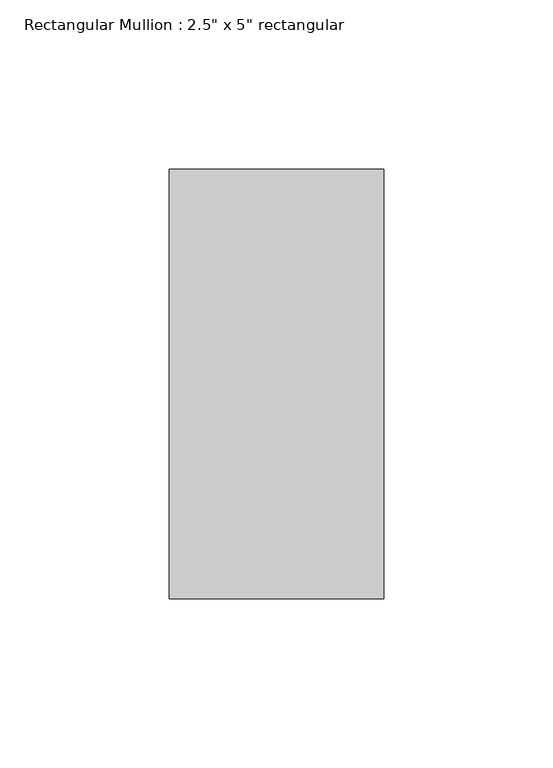
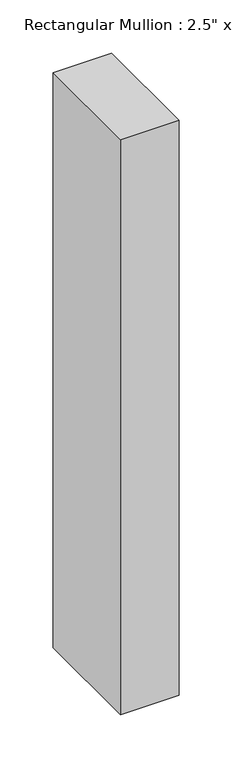
"""IFC4 building model written with IfcOpenShell, lengths in millimetres: member geometry."""

from ifc_helpers import new_model, si_unit, frame, origin, place, context, project, spatial, polyline, outline, extrude, source, transform, mapped, element, save


def member_d3852687(model_context):
    return source(origin(), model_context, "Body", "SweptSolid", [
        extrude(outline(polyline([(0.0, 63.5), (0.0, -63.5), (-63.5, -63.5), (-63.5, 63.5), (0.0, 63.5)])), frame((0.0, 0.0, -660.4), z_axis=(0.0, 0.0, 1.0), x_axis=(1.0, 0.0, 0.0)), (0.0, 0.0, 1.0), 660.4),
    ])


if __name__ == "__main__":
    model = new_model("IFC4")
    model_context = context("Model", 3, world=origin())
    ifc_project = project(units=[si_unit("LENGTHUNIT", "METRE", prefix="MILLI")], contexts=[model_context])
    site = spatial("IfcSite", under=ifc_project)
    building = spatial("IfcBuilding", under=site)
    placement = place(None, origin())
    member_shape = member_d3852687(model_context)
    element("IfcMember", 1, ObjectType="Rectangular Mullion : 2.5\" x 5\" rectangular", at=placement, inside=building, context=model_context, shape_type="MappedRepresentation", body=[
        mapped(member_shape, transform((0.0, 0.0, 0.0), x_axis=(1.0, 0.0, 0.0), y_axis=(0.0, 1.0, 0.0), z_axis=(0.0, 0.0, 1.0))),
    ])
    save(model, "model.ifc")

# Revit data of these elements
# Type "Rectangular Mullion : 2.5\" x 5\" rectangular"
#   built-in parameter 1007304 = 0.416667 (stored number, unit not read)
#   built-in parameter 1007301 = 0.104167 (stored number, unit not read)
#   built-in parameter 1007300 = 0.104167 (stored number, unit not read)
# Element 1 (IfcMember, "Rectangular Mullion : 2.5\" x 5\" rectangular")
#   Materials on its faces: "Aluminum"
# Materials
#   "Aluminum": class "Metal", colour RGB 247 247 247, transparency 0, Description = "Aluminum 6061", Cost = 0
